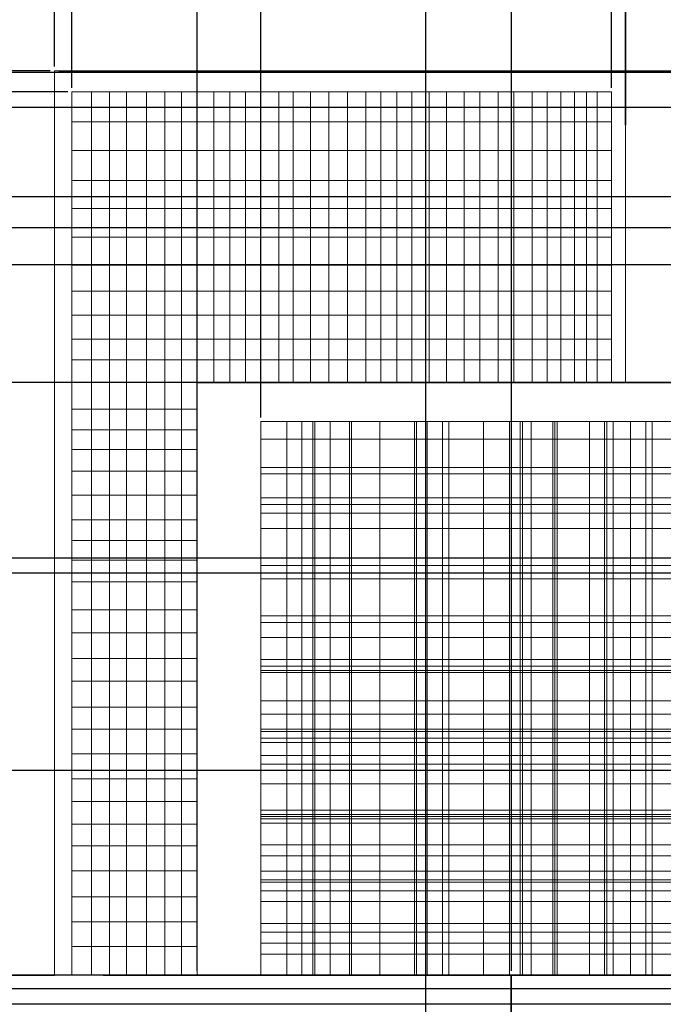
# Model space of a CAD drawing. Units: inches. Extents: x -10 to 130, y -32 to 34.
# Tile 7 of 22: x 19.07 to 28.66, y 5.57 to 20.25. Entities that reach past the tile are written whole.
import ezdxf

# ---------------------------------------------------------------- set-up
doc = ezdxf.new("R2010")
doc.units = ezdxf.units.IN
doc.header["$MEASUREMENT"] = 0
for name, color, linetype, lineweight in [('A-ANNO-DIMS', 2, 'Continuous', 18), ('A-ELEV', 7, 'Continuous', 35), ('A-GLAZ', 4, 'Continuous', 18)]:
    doc.layers.add(name, color=color, linetype=linetype, lineweight=lineweight)
doc.styles.get("Standard").update_dxf_attribs({"font": 'arial.ttf'})
doc.dimstyles.get("Standard").update_dxf_attribs({"dimtxt": 0.18, "dimasz": 0.18, "dimexe": 0.18, "dimexo": 0.0625, "dimgap": 0.09, "dimtad": 0, "dimtih": 1, "dimtoh": 1, "dimdec": 4, "dimzin": 0, "dimdsep": 46, "dimtxsty": 'Standard', "dimcen": 0.09, "dimadec": 0, "dimazin": 0, "dimtfac": 1, "dimtdec": 4, "dimtofl": 0, "dimtmove": 0, "dimatfit": 3, "dimfxl": 1, "dimtolj": 1, "dimtzin": 0, "dimarcsym": 0})

# ---------------------------------------------------------------- blocks, each defined once
blk = doc.blocks.new('*D3')
at = {"layer": 'A-ANNO-DIMS', "color": 0, "lineweight": -2, "transparency": 16777216}
for p, q in [((13.402, 6.07), (13.402, 33.879)), ((21.715, 6.07), (21.715, 33.879)), ((13.582, 33.699), (17.165, 33.699)), ((21.535, 33.699), (17.953, 33.699))]:
    blk.add_line(p, q, dxfattribs=at)
at = {"layer": 'A-ANNO-DIMS', "color": 0, "transparency": 16777216}
for points in [[(13.582, 33.729), (13.582, 33.669), (13.402, 33.699)], [(21.535, 33.729), (21.535, 33.669), (21.715, 33.699)]]:
    blk.add_solid(points, dxfattribs=at)
at = {"layer": 'Defpoints', "color": 0, "transparency": 16777216}
for p in [(21.715, 33.699), (13.402, 6.007), (21.715, 6.007)]:
    blk.add_point(p, dxfattribs=at)
at = {"layer": 'A-ANNO-DIMS', "color": 0, "transparency": 16777216, "insert": (17.559, 33.699), "char_height": 0.18, "attachment_point": 5}
blk.add_mtext('\\A1;8.313', dxfattribs=at)
blk = doc.blocks.new('*D4')
at = {"layer": 'A-ANNO-DIMS', "color": 0, "lineweight": -2, "transparency": 16777216}
for p, q in [((21.715, 6.07), (21.715, 33.879)), ((26.399, 6.07), (26.399, 33.879)), ((21.895, 33.699), (23.66, 33.699)), ((26.219, 33.699), (24.454, 33.699))]:
    blk.add_line(p, q, dxfattribs=at)
at = {"layer": 'A-ANNO-DIMS', "color": 0, "transparency": 16777216}
for points in [[(21.895, 33.729), (21.895, 33.669), (21.715, 33.699)], [(26.219, 33.729), (26.219, 33.669), (26.399, 33.699)]]:
    blk.add_solid(points, dxfattribs=at)
at = {"layer": 'Defpoints', "color": 0, "transparency": 16777216}
for p in [(26.399, 33.699), (21.715, 6.007), (26.399, 6.007)]:
    blk.add_point(p, dxfattribs=at)
at = {"layer": 'A-ANNO-DIMS', "color": 0, "transparency": 16777216, "insert": (24.057, 33.699), "char_height": 0.18, "attachment_point": 5}
blk.add_mtext('\\A1;4.683', dxfattribs=at)
blk = doc.blocks.new('*D5')
at = {"layer": 'A-ANNO-DIMS', "color": 0, "lineweight": -2, "transparency": 16777216}
for p, q in [((26.399, 6.07), (26.399, 33.879)), ((31.971, 6.07), (31.971, 33.879)), ((26.579, 33.699), (28.792, 33.699)), ((31.791, 33.699), (29.578, 33.699))]:
    blk.add_line(p, q, dxfattribs=at)
at = {"layer": 'A-ANNO-DIMS', "color": 0, "transparency": 16777216}
for points in [[(26.579, 33.729), (26.579, 33.669), (26.399, 33.699)], [(31.791, 33.729), (31.791, 33.669), (31.971, 33.699)]]:
    blk.add_solid(points, dxfattribs=at)
at = {"layer": 'Defpoints', "color": 0, "transparency": 16777216}
for p in [(31.971, 33.699), (26.399, 6.007), (31.971, 6.007)]:
    blk.add_point(p, dxfattribs=at)
at = {"layer": 'A-ANNO-DIMS', "color": 0, "transparency": 16777216, "insert": (29.185, 33.699), "char_height": 0.18, "attachment_point": 5}
blk.add_mtext('\\A1;5.572', dxfattribs=at)
blk = doc.blocks.new('*D11')
at = {"layer": 'A-ANNO-DIMS', "color": 0, "lineweight": -2, "transparency": 16777216}
for p, q in [((5.634, -12.739), (5.634, 33.879)), ((19.588, 19.547), (19.588, 33.879)), ((5.814, 33.699), (12.156, 33.699)), ((19.408, 33.699), (13.066, 33.699))]:
    blk.add_line(p, q, dxfattribs=at)
at = {"layer": 'A-ANNO-DIMS', "color": 0, "transparency": 16777216}
for points in [[(5.814, 33.729), (5.814, 33.669), (5.634, 33.699)], [(19.408, 33.729), (19.408, 33.669), (19.588, 33.699)]]:
    blk.add_solid(points, dxfattribs=at)
at = {"layer": 'Defpoints', "color": 0, "transparency": 16777216}
for p in [(19.588, 33.699), (19.588, 19.485), (5.634, -12.801)]:
    blk.add_point(p, dxfattribs=at)
at = {"layer": 'A-ANNO-DIMS', "color": 0, "transparency": 16777216, "insert": (12.611, 33.699), "char_height": 0.18, "attachment_point": 5}
blk.add_mtext('\\A1;13.954', dxfattribs=at)
blk = doc.blocks.new('*D12')
at = {"layer": 'A-ANNO-DIMS', "color": 0, "lineweight": -2, "transparency": 16777216}
for p, q in [((19.588, 19.547), (19.588, 33.879)), ((21.715, 14.903), (21.715, 33.879)), ((19.768, 33.699), (20.326, 33.699)), ((21.535, 33.699), (20.977, 33.699))]:
    blk.add_line(p, q, dxfattribs=at)
at = {"layer": 'A-ANNO-DIMS', "color": 0, "transparency": 16777216}
for points in [[(19.768, 33.729), (19.768, 33.669), (19.588, 33.699)], [(21.535, 33.729), (21.535, 33.669), (21.715, 33.699)]]:
    blk.add_solid(points, dxfattribs=at)
at = {"layer": 'Defpoints', "color": 0, "transparency": 16777216}
for p in [(21.715, 33.699), (19.588, 19.485), (21.715, 14.841)]:
    blk.add_point(p, dxfattribs=at)
at = {"layer": 'A-ANNO-DIMS', "color": 0, "transparency": 16777216, "insert": (20.652, 33.699), "char_height": 0.18, "attachment_point": 5}
blk.add_mtext('\\A1;2.13', dxfattribs=at)
blk = doc.blocks.new('*D13')
at = {"layer": 'A-ANNO-DIMS', "color": 0, "lineweight": -2, "transparency": 16777216}
for p, q in [((21.715, 14.903), (21.715, 33.879)), ((28.1, 24.464), (28.1, 33.879)), ((21.895, 33.699), (24.514, 33.699)), ((27.92, 33.699), (25.301, 33.699))]:
    blk.add_line(p, q, dxfattribs=at)
at = {"layer": 'A-ANNO-DIMS', "color": 0, "transparency": 16777216}
for points in [[(21.895, 33.729), (21.895, 33.669), (21.715, 33.699)], [(27.92, 33.729), (27.92, 33.669), (28.1, 33.699)]]:
    blk.add_solid(points, dxfattribs=at)
at = {"layer": 'Defpoints', "color": 0, "transparency": 16777216}
for p in [(28.1, 33.699), (28.1, 24.402), (21.715, 14.841)]:
    blk.add_point(p, dxfattribs=at)
at = {"layer": 'A-ANNO-DIMS', "color": 0, "transparency": 16777216, "insert": (24.908, 33.699), "char_height": 0.18, "attachment_point": 5}
blk.add_mtext('\\A1;6.384', dxfattribs=at)
blk = doc.blocks.new('*D14')
at = {"layer": 'A-ANNO-DIMS', "color": 0, "lineweight": -2, "transparency": 16777216}
for p, q in [((28.1, 24.464), (28.1, 33.879)), ((33.608, 19.52), (33.608, 33.879)), ((28.28, 33.699), (30.46, 33.699)), ((33.428, 33.699), (31.248, 33.699))]:
    blk.add_line(p, q, dxfattribs=at)
at = {"layer": 'A-ANNO-DIMS', "color": 0, "transparency": 16777216}
for points in [[(28.28, 33.729), (28.28, 33.669), (28.1, 33.699)], [(33.428, 33.729), (33.428, 33.669), (33.608, 33.699)]]:
    blk.add_solid(points, dxfattribs=at)
at = {"layer": 'Defpoints', "color": 0, "transparency": 16777216}
for p in [(33.608, 33.699), (28.1, 24.402), (33.608, 19.458)]:
    blk.add_point(p, dxfattribs=at)
at = {"layer": 'A-ANNO-DIMS', "color": 0, "transparency": 16777216, "insert": (30.854, 33.699), "char_height": 0.18, "attachment_point": 5}
blk.add_mtext('\\A1;5.508', dxfattribs=at)
blk = doc.blocks.new('*D28')
at = {"layer": 'A-ANNO-DIMS', "color": 0, "lineweight": -2, "transparency": 16777216}
for p, q in [((21.715, 14.903), (21.715, 33.879)), ((49.946, 14.903), (49.946, 33.879)), ((21.895, 33.699), (35.436, 33.699)), ((49.766, 33.699), (36.226, 33.699))]:
    blk.add_line(p, q, dxfattribs=at)
at = {"layer": 'A-ANNO-DIMS', "color": 0, "transparency": 16777216}
for points in [[(21.895, 33.729), (21.895, 33.669), (21.715, 33.699)], [(49.766, 33.729), (49.766, 33.669), (49.946, 33.699)]]:
    blk.add_solid(points, dxfattribs=at)
at = {"layer": 'Defpoints', "color": 0, "transparency": 16777216}
for p in [(49.946, 33.699), (21.715, 14.841), (49.946, 14.841)]:
    blk.add_point(p, dxfattribs=at)
at = {"layer": 'A-ANNO-DIMS', "color": 0, "transparency": 16777216, "insert": (35.831, 33.699), "char_height": 0.18, "attachment_point": 5}
blk.add_mtext('\\A1;28.23', dxfattribs=at)
blk = doc.blocks.new('*D34')
at = {"layer": 'A-ANNO-DIMS', "color": 0, "lineweight": -2, "transparency": 16777216}
for p, q in [((13.34, 6.007), (-9.564, 6.007)), ((-9.384, 5.827), (-9.384, 3.941)), ((-9.384, 1.691), (-9.384, 3.577)), ((70.835, 1.511), (-9.564, 1.511))]:
    blk.add_line(p, q, dxfattribs=at)
at = {"layer": 'A-ANNO-DIMS', "color": 0, "transparency": 16777216}
for points in [[(-9.414, 5.827), (-9.354, 5.827), (-9.384, 6.007)], [(-9.414, 1.691), (-9.354, 1.691), (-9.384, 1.511)]]:
    blk.add_solid(points, dxfattribs=at)
at = {"layer": 'Defpoints', "color": 0, "transparency": 16777216}
for p in [(-9.384, 6.007), (13.402, 6.007), (70.898, 1.511)]:
    blk.add_point(p, dxfattribs=at)
at = {"layer": 'A-ANNO-DIMS', "color": 0, "transparency": 16777216, "insert": (-9.384, 3.759), "char_height": 0.18, "attachment_point": 5}
blk.add_mtext('\\A1;4.497', dxfattribs=at)
blk = doc.blocks.new('*D35')
at = {"layer": 'A-ANNO-DIMS', "color": 0, "lineweight": -2, "transparency": 16777216}
for p, q in [((21.653, 14.841), (-9.564, 14.841)), ((-9.384, 14.661), (-9.384, 10.606)), ((-9.384, 6.187), (-9.384, 10.242)), ((13.34, 6.007), (-9.564, 6.007))]:
    blk.add_line(p, q, dxfattribs=at)
at = {"layer": 'A-ANNO-DIMS', "color": 0, "transparency": 16777216}
for points in [[(-9.414, 14.661), (-9.354, 14.661), (-9.384, 14.841)], [(-9.414, 6.187), (-9.354, 6.187), (-9.384, 6.007)]]:
    blk.add_solid(points, dxfattribs=at)
at = {"layer": 'Defpoints', "color": 0, "transparency": 16777216}
for p in [(-9.384, 14.841), (21.715, 14.841), (13.402, 6.007)]:
    blk.add_point(p, dxfattribs=at)
at = {"layer": 'A-ANNO-DIMS', "color": 0, "transparency": 16777216, "insert": (-9.384, 10.424), "char_height": 0.18, "attachment_point": 5}
blk.add_mtext('\\A1;8.833', dxfattribs=at)
blk = doc.blocks.new('*D36')
at = {"layer": 'A-ANNO-DIMS', "color": 0, "lineweight": -2, "transparency": 16777216}
for p, q in [((44.559, 17.607), (-9.564, 17.607)), ((-9.384, 17.427), (-9.384, 16.405)), ((-9.384, 15.021), (-9.384, 16.044)), ((21.653, 14.841), (-9.564, 14.841))]:
    blk.add_line(p, q, dxfattribs=at)
at = {"layer": 'A-ANNO-DIMS', "color": 0, "transparency": 16777216}
for points in [[(-9.414, 17.427), (-9.354, 17.427), (-9.384, 17.607)], [(-9.414, 15.021), (-9.354, 15.021), (-9.384, 14.841)]]:
    blk.add_solid(points, dxfattribs=at)
at = {"layer": 'Defpoints', "color": 0, "transparency": 16777216}
for p in [(-9.384, 17.607), (44.622, 17.607), (21.715, 14.841)]:
    blk.add_point(p, dxfattribs=at)
at = {"layer": 'A-ANNO-DIMS', "color": 0, "transparency": 16777216, "insert": (-9.384, 16.224), "char_height": 0.18, "attachment_point": 5}
blk.add_mtext('\\A1;2.77', dxfattribs=at)
blk = doc.blocks.new('*D37')
at = {"layer": 'A-ANNO-DIMS', "color": 0, "lineweight": -2, "transparency": 16777216}
for p, q in [((19.526, 19.485), (-9.564, 19.485)), ((-9.384, 19.305), (-9.384, 18.728)), ((-9.384, 17.787), (-9.384, 18.364)), ((44.559, 17.607), (-9.564, 17.607))]:
    blk.add_line(p, q, dxfattribs=at)
at = {"layer": 'A-ANNO-DIMS', "color": 0, "transparency": 16777216}
for points in [[(-9.414, 19.305), (-9.354, 19.305), (-9.384, 19.485)], [(-9.414, 17.787), (-9.354, 17.787), (-9.384, 17.607)]]:
    blk.add_solid(points, dxfattribs=at)
at = {"layer": 'Defpoints', "color": 0, "transparency": 16777216}
for p in [(-9.384, 19.485), (19.588, 19.485), (44.622, 17.607)]:
    blk.add_point(p, dxfattribs=at)
at = {"layer": 'A-ANNO-DIMS', "color": 0, "transparency": 16777216, "insert": (-9.384, 18.546), "char_height": 0.18, "attachment_point": 5}
blk.add_mtext('\\A1;1.877', dxfattribs=at)
blk = doc.blocks.new('*D38')
at = {"layer": 'A-ANNO-DIMS', "color": 0, "lineweight": -2, "transparency": 16777216}
for p, q in [((28.037, 24.402), (-9.564, 24.402)), ((-9.384, 24.222), (-9.384, 22.125)), ((-9.384, 19.665), (-9.384, 21.761)), ((19.526, 19.485), (-9.564, 19.485))]:
    blk.add_line(p, q, dxfattribs=at)
at = {"layer": 'A-ANNO-DIMS', "color": 0, "transparency": 16777216}
for points in [[(-9.414, 24.222), (-9.354, 24.222), (-9.384, 24.402)], [(-9.414, 19.665), (-9.354, 19.665), (-9.384, 19.485)]]:
    blk.add_solid(points, dxfattribs=at)
at = {"layer": 'Defpoints', "color": 0, "transparency": 16777216}
for p in [(-9.384, 24.402), (28.1, 24.402), (19.588, 19.485)]:
    blk.add_point(p, dxfattribs=at)
at = {"layer": 'A-ANNO-DIMS', "color": 0, "transparency": 16777216, "insert": (-9.384, 21.943), "char_height": 0.18, "attachment_point": 5}
blk.add_mtext('\\A1;4.917', dxfattribs=at)
blk = doc.blocks.new('*D74')
at = {"layer": 'A-ANNO-DIMS', "color": 0, "lineweight": -2, "transparency": 16777216}
for p, q in [((54.085, 17.607), (-9.564, 17.607)), ((-9.384, 17.427), (-9.384, 17.281)), ((-9.384, 16.771), (-9.384, 16.917)), ((55.856, 16.591), (-9.564, 16.591))]:
    blk.add_line(p, q, dxfattribs=at)
at = {"layer": 'A-ANNO-DIMS', "color": 0, "transparency": 16777216}
for points in [[(-9.414, 17.427), (-9.354, 17.427), (-9.384, 17.607)], [(-9.414, 16.771), (-9.354, 16.771), (-9.384, 16.591)]]:
    blk.add_solid(points, dxfattribs=at)
at = {"layer": 'Defpoints', "color": 0, "transparency": 16777216}
for p in [(54.147, 17.607), (-9.384, 16.591), (55.918, 16.591)]:
    blk.add_point(p, dxfattribs=at)
at = {"layer": 'A-ANNO-DIMS', "color": 0, "transparency": 16777216, "insert": (-9.384, 17.099), "char_height": 0.18, "attachment_point": 5}
blk.add_mtext('\\A1;1.02', dxfattribs=at)
blk = doc.blocks.new('*D82')
at = {"layer": 'A-ANNO-DIMS', "color": 0, "lineweight": -2, "transparency": 16777216}
for p, q in [((19.651, 19.485), (129.508, 19.485)), ((129.328, 19.305), (129.328, 18.728)), ((129.328, 17.787), (129.328, 18.364)), ((68.738, 17.607), (129.508, 17.607))]:
    blk.add_line(p, q, dxfattribs=at)
at = {"layer": 'A-ANNO-DIMS', "color": 0, "transparency": 16777216}
for points in [[(129.298, 19.305), (129.358, 19.305), (129.328, 19.485)], [(129.298, 17.787), (129.358, 17.787), (129.328, 17.607)]]:
    blk.add_solid(points, dxfattribs=at)
at = {"layer": 'Defpoints', "color": 0, "transparency": 16777216}
for p in [(19.588, 19.485), (68.676, 17.607), (129.328, 17.607)]:
    blk.add_point(p, dxfattribs=at)
at = {"layer": 'A-ANNO-DIMS', "color": 0, "transparency": 16777216, "insert": (129.328, 18.546), "char_height": 0.18, "attachment_point": 5}
blk.add_mtext('\\A1;1.877', dxfattribs=at)
blk = doc.blocks.new('*D87')
at = {"layer": 'A-ANNO-DIMS', "color": 0, "lineweight": -2, "transparency": 16777216}
for p, q in [((49.884, 14.841), (-9.564, 14.841)), ((-9.384, 14.661), (-9.384, 13.713)), ((-9.384, 12.402), (-9.384, 13.35)), ((49.884, 12.222), (-9.564, 12.222))]:
    blk.add_line(p, q, dxfattribs=at)
at = {"layer": 'A-ANNO-DIMS', "color": 0, "transparency": 16777216}
for points in [[(-9.414, 14.661), (-9.354, 14.661), (-9.384, 14.841)], [(-9.414, 12.402), (-9.354, 12.402), (-9.384, 12.222)]]:
    blk.add_solid(points, dxfattribs=at)
at = {"layer": 'Defpoints', "color": 0, "transparency": 16777216}
for p in [(49.946, 14.841), (-9.384, 12.222), (49.946, 12.222)]:
    blk.add_point(p, dxfattribs=at)
at = {"layer": 'A-ANNO-DIMS', "color": 0, "transparency": 16777216, "insert": (-9.384, 13.532), "char_height": 0.18, "attachment_point": 5}
blk.add_mtext('\\A1;2.619', dxfattribs=at)
blk = doc.blocks.new('*D88')
at = {"layer": 'A-ANNO-DIMS', "color": 0, "lineweight": -2, "transparency": 16777216}
for p, q in [((49.884, 12.222), (-9.564, 12.222)), ((-9.384, 12.042), (-9.384, 10.822)), ((-9.384, 9.238), (-9.384, 10.458)), ((49.884, 9.058), (-9.564, 9.058))]:
    blk.add_line(p, q, dxfattribs=at)
at = {"layer": 'A-ANNO-DIMS', "color": 0, "transparency": 16777216}
for points in [[(-9.414, 12.042), (-9.354, 12.042), (-9.384, 12.222)], [(-9.414, 9.238), (-9.354, 9.238), (-9.384, 9.058)]]:
    blk.add_solid(points, dxfattribs=at)
at = {"layer": 'Defpoints', "color": 0, "transparency": 16777216}
for p in [(49.946, 12.222), (-9.384, 9.058), (49.946, 9.058)]:
    blk.add_point(p, dxfattribs=at)
at = {"layer": 'A-ANNO-DIMS', "color": 0, "transparency": 16777216, "insert": (-9.384, 10.64), "char_height": 0.18, "attachment_point": 5}
blk.add_mtext('\\A1;3.164', dxfattribs=at)
blk = doc.blocks.new('*D89')
at = {"layer": 'A-ANNO-DIMS', "color": 0, "lineweight": -2, "transparency": 16777216}
for p, q in [((49.884, 9.058), (-9.564, 9.058)), ((-9.384, 8.878), (-9.384, 7.612)), ((-9.384, 5.982), (-9.384, 7.248)), ((49.884, 5.802), (-9.564, 5.802))]:
    blk.add_line(p, q, dxfattribs=at)
at = {"layer": 'A-ANNO-DIMS', "color": 0, "transparency": 16777216}
for points in [[(-9.414, 8.878), (-9.354, 8.878), (-9.384, 9.058)], [(-9.414, 5.982), (-9.354, 5.982), (-9.384, 5.802)]]:
    blk.add_solid(points, dxfattribs=at)
at = {"layer": 'Defpoints', "color": 0, "transparency": 16777216}
for p in [(49.946, 9.058), (-9.384, 5.802), (49.946, 5.802)]:
    blk.add_point(p, dxfattribs=at)
at = {"layer": 'A-ANNO-DIMS', "color": 0, "transparency": 16777216, "insert": (-9.384, 7.43), "char_height": 0.18, "attachment_point": 5}
blk.add_mtext('\\A1;3.256', dxfattribs=at)
blk = doc.blocks.new('*D90')
at = {"layer": 'A-ANNO-DIMS', "color": 0, "lineweight": -2, "transparency": 16777216}
for p, q in [((49.884, 5.802), (-9.564, 5.802)), ((-9.384, 5.622), (-9.384, 4.421)), ((-9.384, 2.855), (-9.384, 4.057)), ((49.884, 2.675), (-9.564, 2.675))]:
    blk.add_line(p, q, dxfattribs=at)
at = {"layer": 'A-ANNO-DIMS', "color": 0, "transparency": 16777216}
for points in [[(-9.414, 5.622), (-9.354, 5.622), (-9.384, 5.802)], [(-9.414, 2.855), (-9.354, 2.855), (-9.384, 2.675)]]:
    blk.add_solid(points, dxfattribs=at)
at = {"layer": 'Defpoints', "color": 0, "transparency": 16777216}
for p in [(49.946, 5.802), (-9.384, 2.675), (49.946, 2.675)]:
    blk.add_point(p, dxfattribs=at)
at = {"layer": 'A-ANNO-DIMS', "color": 0, "transparency": 16777216, "insert": (-9.384, 4.239), "char_height": 0.18, "attachment_point": 5}
blk.add_mtext('\\A1;3.127', dxfattribs=at)
blk = doc.blocks.new('*D95')
at = {"layer": 'A-ANNO-DIMS', "color": 0, "lineweight": -2, "transparency": 16777216}
for p, q in [((-9.384, 12.402), (-9.384, 12.582)), ((49.884, 12.222), (-9.564, 12.222)), ((49.884, 11.995), (-9.564, 11.995)), ((-9.384, 11.815), (-9.384, 11.635)), ((-9.384, 11.635), (-9.564, 11.635))]:
    blk.add_line(p, q, dxfattribs=at)
at = {"layer": 'A-ANNO-DIMS', "color": 0, "transparency": 16777216}
for points in [[(-9.414, 12.402), (-9.354, 12.402), (-9.384, 12.222)], [(-9.414, 11.815), (-9.354, 11.815), (-9.384, 11.995)]]:
    blk.add_solid(points, dxfattribs=at)
at = {"layer": 'Defpoints', "color": 0, "transparency": 16777216}
for p in [(49.946, 12.222), (-9.384, 11.995), (49.946, 11.995)]:
    blk.add_point(p, dxfattribs=at)
at = {"layer": 'A-ANNO-DIMS', "color": 0, "transparency": 16777216, "insert": (-9.957, 11.635), "char_height": 0.18, "attachment_point": 5}
blk.add_mtext('\\A1;0.227', dxfattribs=at)
blk = doc.blocks.new('*D96')
at = {"layer": 'A-ANNO-DIMS', "color": 0, "lineweight": -2, "transparency": 16777216}
for p, q in [((19.588, 19.547), (19.588, 33.879)), ((19.848, 19.232), (19.848, 33.879)), ((19.408, 33.699), (19.228, 33.699)), ((20.028, 33.699), (20.208, 33.699))]:
    blk.add_line(p, q, dxfattribs=at)
at = {"layer": 'A-ANNO-DIMS', "color": 0, "transparency": 16777216}
for points in [[(19.408, 33.729), (19.408, 33.669), (19.588, 33.699)], [(20.028, 33.729), (20.028, 33.669), (19.848, 33.699)]]:
    blk.add_solid(points, dxfattribs=at)
at = {"layer": 'Defpoints', "color": 0, "transparency": 16777216}
for p in [(19.848, 33.699), (19.588, 19.485), (19.848, 19.17)]:
    blk.add_point(p, dxfattribs=at)
at = {"layer": 'A-ANNO-DIMS', "color": 0, "transparency": 16777216, "insert": (20.601, 33.699), "char_height": 0.18, "attachment_point": 5}
blk.add_mtext('\\A1;0.260', dxfattribs=at)
blk = doc.blocks.new('*D97')
at = {"layer": 'A-ANNO-DIMS', "color": 0, "lineweight": -2, "transparency": 16777216}
for p, q in [((19.848, 19.232), (19.848, 33.879)), ((27.892, 19.232), (27.892, 33.879)), ((20.028, 33.699), (23.476, 33.699)), ((27.712, 33.699), (24.263, 33.699))]:
    blk.add_line(p, q, dxfattribs=at)
at = {"layer": 'A-ANNO-DIMS', "color": 0, "transparency": 16777216}
for points in [[(20.028, 33.729), (20.028, 33.669), (19.848, 33.699)], [(27.712, 33.729), (27.712, 33.669), (27.892, 33.699)]]:
    blk.add_solid(points, dxfattribs=at)
at = {"layer": 'Defpoints', "color": 0, "transparency": 16777216}
for p in [(27.892, 33.699), (19.848, 19.17), (27.892, 19.17)]:
    blk.add_point(p, dxfattribs=at)
at = {"layer": 'A-ANNO-DIMS', "color": 0, "transparency": 16777216, "insert": (23.87, 33.699), "char_height": 0.18, "attachment_point": 5}
blk.add_mtext('\\A1;8.044', dxfattribs=at)
blk = doc.blocks.new('*D98')
at = {"layer": 'A-ANNO-DIMS', "color": 0, "lineweight": -2, "transparency": 16777216}
for p, q in [((-9.384, 19.665), (-9.384, 19.845)), ((-9.384, 19.845), (-9.204, 19.845)), ((19.526, 19.485), (-9.564, 19.485)), ((19.785, 19.17), (-9.564, 19.17)), ((-9.384, 18.99), (-9.384, 18.81))]:
    blk.add_line(p, q, dxfattribs=at)
at = {"layer": 'A-ANNO-DIMS', "color": 0, "transparency": 16777216}
for points in [[(-9.414, 19.665), (-9.354, 19.665), (-9.384, 19.485)], [(-9.414, 18.99), (-9.354, 18.99), (-9.384, 19.17)]]:
    blk.add_solid(points, dxfattribs=at)
at = {"layer": 'Defpoints', "color": 0, "transparency": 16777216}
for p in [(-9.384, 19.485), (19.588, 19.485), (19.848, 19.17)]:
    blk.add_point(p, dxfattribs=at)
at = {"layer": 'A-ANNO-DIMS', "color": 0, "transparency": 16777216, "insert": (-8.809, 19.845), "char_height": 0.18, "attachment_point": 5}
blk.add_mtext('\\A1;0.315', dxfattribs=at)
blk = doc.blocks.new('*D104')
at = {"layer": 'A-ANNO-DIMS', "color": 0, "lineweight": -2, "transparency": 16777216}
for p, q in [((-9.383551, 19.637521), (-9.383551, 19.817521)), ((33.54566, 19.457521), (-9.563551, 19.457521)), ((33.931459, 18.935883), (-9.563551, 18.935883)), ((-9.383551, 18.755883), (-9.383551, 18.575883))]:
    blk.add_line(p, q, dxfattribs=at)
at = {"layer": 'A-ANNO-DIMS', "color": 0, "transparency": 16777216}
for points in [[(-9.413551, 19.637521), (-9.353551, 19.637521), (-9.383551, 19.457521)], [(-9.413551, 18.755883), (-9.353551, 18.755883), (-9.383551, 18.935883)]]:
    blk.add_solid(points, dxfattribs=at)
at = {"layer": 'Defpoints', "color": 0, "transparency": 16777216}
for p in [(-9.383551, 19.457521), (33.60816, 19.457521), (33.993959, 18.935883)]:
    blk.add_point(p, dxfattribs=at)
at = {"layer": 'A-ANNO-DIMS', "color": 0, "transparency": 16777216, "insert": (-9.383551, 19.196702), "char_height": 0.18, "attachment_point": 5}
blk.add_mtext('\\A1;0.522', dxfattribs=at)
blk = doc.blocks.new('*D105')
at = {"layer": 'A-ANNO-DIMS', "color": 0, "lineweight": -2, "transparency": 16777216}
for p, q in [((21.715452, 14.90344), (21.715452, 33.878656)), ((22.664856, 14.318095), (22.664856, 33.878656)), ((21.535452, 33.698656), (21.355452, 33.698656)), ((22.844856, 33.698656), (23.024856, 33.698656))]:
    blk.add_line(p, q, dxfattribs=at)
at = {"layer": 'A-ANNO-DIMS', "color": 0, "transparency": 16777216}
for points in [[(21.535452, 33.728656), (21.535452, 33.668656), (21.715452, 33.698656)], [(22.844856, 33.728656), (22.844856, 33.668656), (22.664856, 33.698656)]]:
    blk.add_solid(points, dxfattribs=at)
at = {"layer": 'Defpoints', "color": 0, "transparency": 16777216}
for p in [(22.664856, 33.698656), (21.715452, 14.84094), (22.664856, 14.255595)]:
    blk.add_point(p, dxfattribs=at)
at = {"layer": 'A-ANNO-DIMS', "color": 0, "transparency": 16777216, "insert": (22.190154, 33.698656), "char_height": 0.18, "attachment_point": 5}
blk.add_mtext('\\A1;0.949', dxfattribs=at)
blk = doc.blocks.new('*D106')
at = {"layer": 'A-ANNO-DIMS', "color": 0, "lineweight": -2, "transparency": 16777216}
for p, q in [((22.665, 14.318), (22.665, 33.879)), ((48.963, 14.318), (48.963, 33.879)), ((22.845, 33.699), (35.349, 33.699)), ((48.783, 33.699), (36.279, 33.699))]:
    blk.add_line(p, q, dxfattribs=at)
at = {"layer": 'A-ANNO-DIMS', "color": 0, "transparency": 16777216}
for points in [[(22.845, 33.729), (22.845, 33.669), (22.665, 33.699)], [(48.783, 33.729), (48.783, 33.669), (48.963, 33.699)]]:
    blk.add_solid(points, dxfattribs=at)
at = {"layer": 'Defpoints', "color": 0, "transparency": 16777216}
for p in [(48.963, 33.699), (22.665, 14.256), (48.963, 14.256)]:
    blk.add_point(p, dxfattribs=at)
at = {"layer": 'A-ANNO-DIMS', "color": 0, "transparency": 16777216, "insert": (35.814, 33.699), "char_height": 0.18, "attachment_point": 5}
blk.add_mtext('\\A1;26.298', dxfattribs=at)
blk = doc.blocks.new('*D110')
at = {"layer": 'A-ANNO-DIMS', "color": 0, "lineweight": -2, "transparency": 16777216}
for p, q in [((-9.383551, 17.787359), (-9.383551, 17.967359)), ((44.559228, 17.607359), (-9.563551, 17.607359)), ((45.040057, 17.142679), (-9.563551, 17.142679)), ((-9.383551, 16.962679), (-9.383551, 16.782679))]:
    blk.add_line(p, q, dxfattribs=at)
at = {"layer": 'A-ANNO-DIMS', "color": 0, "transparency": 16777216}
for points in [[(-9.413551, 17.787359), (-9.353551, 17.787359), (-9.383551, 17.607359)], [(-9.413551, 16.962679), (-9.353551, 16.962679), (-9.383551, 17.142679)]]:
    blk.add_solid(points, dxfattribs=at)
at = {"layer": 'Defpoints', "color": 0, "transparency": 16777216}
for p in [(-9.383551, 17.607359), (44.621728, 17.607359), (45.102557, 17.142679)]:
    blk.add_point(p, dxfattribs=at)
at = {"layer": 'A-ANNO-DIMS', "color": 0, "transparency": 16777216, "insert": (-9.383551, 17.375019), "char_height": 0.18, "attachment_point": 5}
blk.add_mtext('\\A1;0.465', dxfattribs=at)
blk = doc.blocks.new('*D112')
at = {"layer": 'A-ANNO-DIMS', "color": 0, "lineweight": -2, "transparency": 16777216}
for p, q in [((14.732, 5.012), (14.732, 33.879)), ((25.126, 5.012), (25.126, 33.879)), ((14.912, 33.699), (19.474, 33.699)), ((24.946, 33.699), (20.384, 33.699))]:
    blk.add_line(p, q, dxfattribs=at)
at = {"layer": 'A-ANNO-DIMS', "color": 0, "transparency": 16777216}
for points in [[(14.912, 33.729), (14.912, 33.669), (14.732, 33.699)], [(24.946, 33.729), (24.946, 33.669), (25.126, 33.699)]]:
    blk.add_solid(points, dxfattribs=at)
at = {"layer": 'Defpoints', "color": 0, "transparency": 16777216}
for p in [(25.126, 33.699), (14.732, 4.95), (25.126, 4.95)]:
    blk.add_point(p, dxfattribs=at)
at = {"layer": 'A-ANNO-DIMS', "color": 0, "transparency": 16777216, "insert": (19.929, 33.699), "char_height": 0.18, "attachment_point": 5}
blk.add_mtext('\\A1;10.394', dxfattribs=at)
blk = doc.blocks.new('*D115')
at = {"layer": 'A-ANNO-DIMS', "color": 0, "lineweight": -2, "transparency": 16777216}
for p, q in [((26.336, 6.007), (-9.564, 6.007)), ((-9.384, 5.827), (-9.384, 4.151)), ((-9.384, 2.111), (-9.384, 3.787)), ((26.336, 1.931), (-9.564, 1.931))]:
    blk.add_line(p, q, dxfattribs=at)
at = {"layer": 'A-ANNO-DIMS', "color": 0, "transparency": 16777216}
for points in [[(-9.414, 5.827), (-9.354, 5.827), (-9.384, 6.007)], [(-9.414, 2.111), (-9.354, 2.111), (-9.384, 1.931)]]:
    blk.add_solid(points, dxfattribs=at)
at = {"layer": 'Defpoints', "color": 0, "transparency": 16777216}
for p in [(26.399, 6.007), (-9.384, 1.931), (26.399, 1.931)]:
    blk.add_point(p, dxfattribs=at)
at = {"layer": 'A-ANNO-DIMS', "color": 0, "transparency": 16777216, "insert": (-9.384, 3.969), "char_height": 0.18, "attachment_point": 5}
blk.add_mtext('\\A1;4.076', dxfattribs=at)
blk = doc.blocks.new('*D121')
at = {"layer": 'A-ANNO-DIMS', "color": 0, "lineweight": -2, "transparency": 16777216}
for p, q in [((-9.384, 6.187), (-9.384, 6.367)), ((31.909, 6.007), (-9.564, 6.007)), ((32.427, 5.572), (-9.564, 5.572)), ((-9.384, 5.392), (-9.384, 5.212))]:
    blk.add_line(p, q, dxfattribs=at)
at = {"layer": 'A-ANNO-DIMS', "color": 0, "transparency": 16777216}
for points in [[(-9.414, 6.187), (-9.354, 6.187), (-9.384, 6.007)], [(-9.414, 5.392), (-9.354, 5.392), (-9.384, 5.572)]]:
    blk.add_solid(points, dxfattribs=at)
at = {"layer": 'Defpoints', "color": 0, "transparency": 16777216}
for p in [(-9.384, 6.007), (31.971, 6.007), (32.49, 5.572)]:
    blk.add_point(p, dxfattribs=at)
at = {"layer": 'A-ANNO-DIMS', "color": 0, "transparency": 16777216, "insert": (-9.384, 5.789), "char_height": 0.18, "attachment_point": 5}
blk.add_mtext('\\A1;0.436', dxfattribs=at)

msp = doc.modelspace()

# ---------------------------------------------------------------- linework, layer by layer
at = {"layer": 'A-ELEV'}
for p, q in [((28.0997, 18.6807), (28.0997, 24.4019)), ((21.7155, 14.8409), (49.9462, 14.8409)), ((19.5881, 6.0074), (13.4021, 6.0074)), ((20.3124, 6.0074), (49.9462, 6.0074)), ((26.3988, -6.2218), (26.3988, 6.0074))]:
    msp.add_line(p, q, dxfattribs=at)
at = {"layer": 'A-GLAZ'}
for p, q in [((20.3124, 19.4845), (19.5881, 19.4845)), ((19.5881, 19.4845), (19.5881, 18.6807)), ((20.3124, 19.4845), (28.0997, 19.4845)), ((19.8477, 19.1697), (27.8916, 19.1697)), ((19.8477, 19.1697), (19.8477, 18.6807)), ((20.1415, 19.1697), (20.1415, 18.6807)), ((20.408, 19.1697), (20.408, 18.6807)), ((20.6608, 19.1697), (20.6608, 18.6807)), ((20.9614, 19.1697), (20.9614, 18.6807)), ((21.2347, 19.1697), (21.2347, 18.6807)), ((21.4807, 19.1697), (21.4807, 18.6807)), ((21.7155, 14.8409), (21.7155, 19.1697)), ((21.9634, 14.8409), (21.9634, 19.1697)), ((22.2001, 14.8409), (22.2001, 19.1697)), ((22.4368, 14.8409), (22.4368, 19.1697)), ((22.6622, 14.8409), (22.6622, 19.1697)), ((22.9326, 14.8409), (22.9326, 19.1697)), ((23.1468, 14.8409), (23.1468, 19.1697)), ((23.406, 14.8409), (23.406, 19.1697)), ((23.6765, 14.8409), (23.6765, 19.1697)), ((23.9582, 14.8409), (23.9582, 19.1697)), ((24.2287, 14.8409), (24.2287, 19.1697)), ((24.4541, 14.8409), (24.4541, 19.1697)), ((24.6908, 14.8409), (24.6908, 19.1697)), ((24.9162, 14.8409), (24.9162, 19.1697)), ((25.1754, 14.8409), (25.1754, 19.1697)), ((25.4346, 14.8409), (25.4346, 19.1697)), ((25.6939, 14.8409), (25.6939, 19.1697)), ((25.9305, 14.8409), (25.9305, 19.1697)), ((26.201, 14.8409), (26.201, 19.1697)), ((26.4377, 14.8409), (26.4377, 19.1697)), ((26.7082, 14.8409), (26.7082, 19.1697)), ((26.9336, 14.8409), (26.9336, 19.1697)), ((27.1365, 14.8409), (27.1365, 19.1697)), ((27.3393, 14.8409), (27.3393, 19.1697)), ((27.5197, 14.8409), (27.5197, 19.1697)), ((27.6774, 14.8409), (27.6774, 19.1697)), ((27.8916, 14.8409), (27.8916, 19.1697)), ((19.5881, 18.6807), (19.5881, 6.7976)), ((19.8477, 18.7245), (27.8916, 18.7245)), ((19.8477, 18.6807), (19.8477, 6.7976)), ((20.1415, 18.6807), (20.1415, 6.7976)), ((20.408, 18.6807), (20.408, 6.7976)), ((20.6608, 18.6807), (20.6608, 6.7976)), ((20.9614, 18.6807), (20.9614, 6.7976)), ((21.2347, 18.6807), (21.2347, 6.7976)), ((21.4807, 18.6807), (21.4807, 6.7976)), ((28.0997, 18.6807), (28.0997, 14.8409)), ((20.3124, 18.2941), (19.8477, 18.2941)), ((20.3124, 18.2941), (27.8916, 18.2941)), ((20.3124, 17.8489), (19.8477, 17.8489)), ((20.3124, 17.8489), (27.8916, 17.8489)), ((20.3124, 17.4334), (19.8477, 17.4334)), ((20.3124, 17.4334), (27.8916, 17.4334)), ((20.3124, 17.0031), (19.8477, 17.0031)), ((20.3124, 17.0031), (27.8916, 17.0031)), ((20.3124, 16.5876), (19.8477, 16.5876)), ((20.3124, 16.5876), (27.8916, 16.5876)), ((20.3124, 16.1986), (19.8477, 16.1986)), ((20.3124, 16.1986), (27.8916, 16.1986)), ((20.3124, 15.8424), (19.8477, 15.8424)), ((20.3124, 15.8424), (27.8916, 15.8424)), ((20.3124, 15.4863), (19.8477, 15.4863)), ((20.3124, 15.4863), (27.8916, 15.4863)), ((20.3124, 15.1746), (19.8477, 15.1746)), ((20.3124, 15.1746), (27.8916, 15.1746)), ((21.7155, 14.8409), (19.8477, 14.8409)), ((21.7155, 6.0074), (21.7155, 14.8409)), ((20.3124, 14.4405), (19.8477, 14.4405)), ((20.3124, 14.4405), (21.7155, 14.4405)), ((22.6649, 6.0074), (22.6649, 14.2556)), ((22.6649, 14.2556), (48.963, 14.2556)), ((23.0516, 6.0074), (23.0516, 14.2556)), ((23.2772, 6.0074), (23.2772, 14.2556)), ((23.4383, 6.0074), (23.4383, 14.2556)), ((23.4706, 6.0074), (23.4706, 14.2556)), ((23.6962, 6.0074), (23.6962, 14.2556)), ((23.9862, 6.0074), (23.9862, 14.2556)), ((24.0184, 6.0074), (24.0184, 14.2556)), ((24.4374, 6.0074), (24.4374, 14.2556)), ((24.9531, 6.0074), (24.9531, 14.2556)), ((24.9853, 6.0074), (24.9853, 14.2556)), ((25.1464, 6.0074), (25.1464, 14.2556)), ((25.372, 6.0074), (25.372, 14.2556)), ((25.4687, 6.0074), (25.4687, 14.2556)), ((25.4687, 6.0074), (25.4687, 14.2556)), ((25.9844, 6.0074), (25.9844, 14.2556)), ((25.9844, 6.0074), (25.9844, 14.2556)), ((26.3711, 6.0074), (26.3711, 14.2556)), ((26.5322, 6.0074), (26.5322, 14.2556)), ((26.5645, 6.0074), (26.5645, 14.2556)), ((26.6934, 6.0074), (26.6934, 14.2556)), ((27.0156, 6.0074), (27.0156, 14.2556)), ((27.0479, 6.0074), (27.0479, 14.2556)), ((27.0801, 6.0074), (27.0801, 14.2556)), ((27.5635, 6.0074), (27.5635, 14.2556)), ((27.7891, 6.0074), (27.7891, 14.2556)), ((27.8214, 6.0074), (27.8214, 14.2556)), ((27.918, 6.0074), (27.918, 14.2556)), ((28.1759, 6.0074), (28.1759, 14.2556)), ((28.4015, 6.0074), (28.4015, 14.2556)), ((28.4981, 6.0074), (28.4981, 14.2556)), ((20.3124, 14.1324), (19.8477, 14.1324)), ((20.3124, 14.1324), (21.7155, 14.1324)), ((22.6649, 13.9954), (48.963, 13.9954)), ((20.3124, 13.8397), (19.8477, 13.8397)), ((20.3124, 13.8397), (21.7155, 13.8397)), ((20.3124, 13.5162), (19.8477, 13.5162)), ((20.3124, 13.5162), (21.7155, 13.5162)), ((22.6649, 13.5727), (48.963, 13.5727)), ((22.6649, 13.4751), (48.963, 13.4751)), ((20.3124, 13.1619), (19.8477, 13.1619)), ((20.3124, 13.1619), (21.7155, 13.1619)), ((22.6649, 13.1174), (48.963, 13.1174)), ((22.6649, 13.0199), (48.963, 13.0199)), ((20.3124, 12.7922), (19.8477, 12.7922)), ((20.3124, 12.7922), (21.7155, 12.7922)), ((22.6649, 12.8898), (48.963, 12.8898)), ((22.6649, 12.8898), (48.963, 12.8898)), ((22.6649, 12.6622), (48.963, 12.6622)), ((20.3124, 12.4841), (19.8477, 12.4841)), ((20.3124, 12.4841), (21.7155, 12.4841)), ((20.3124, 12.1914), (19.8477, 12.1914)), ((20.3124, 12.1914), (21.7155, 12.1914)), ((22.6649, 12.1093), (48.963, 12.1093)), ((22.6649, 11.9142), (48.963, 11.9142)), ((20.3124, 11.8679), (19.8477, 11.8679)), ((20.3124, 11.8679), (21.7155, 11.8679)), ((20.3124, 11.4484), (19.8477, 11.4484)), ((20.3124, 11.4484), (21.7155, 11.4484)), ((22.6649, 11.3614), (48.963, 11.3614)), ((22.6649, 11.3614), (48.963, 11.3614)), ((22.6649, 11.2638), (48.963, 11.2638)), ((20.3124, 11.1095), (19.8477, 11.1095)), ((20.3124, 11.1095), (21.7155, 11.1095)), ((22.6649, 11.0362), (48.963, 11.0362)), ((20.3124, 10.7244), (19.8477, 10.7244)), ((20.3124, 10.7244), (21.7155, 10.7244)), ((22.6649, 10.711), (48.963, 10.711)), ((22.6649, 10.711), (48.963, 10.711)), ((22.6649, 10.711), (48.963, 10.711)), ((22.6649, 10.6134), (48.963, 10.6134)), ((22.6649, 10.5484), (48.963, 10.5484)), ((22.6649, 10.5159), (48.963, 10.5159)), ((20.3124, 10.3855), (19.8477, 10.3855)), ((20.3124, 10.3855), (21.7155, 10.3855)), ((20.3124, 10.0004), (19.8477, 10.0004)), ((20.3124, 10.0004), (21.7155, 10.0004)), ((22.6649, 10.0931), (48.963, 10.0931)), ((22.6649, 9.898), (48.963, 9.898)), ((20.3124, 9.6726), (19.8477, 9.6726)), ((20.3124, 9.6726), (21.7155, 9.6726)), ((22.6649, 9.6704), (48.963, 9.6704)), ((22.6649, 9.6379), (48.963, 9.6379)), ((22.6649, 9.5403), (48.963, 9.5403)), ((22.6649, 9.4753), (48.963, 9.4753)), ((20.3124, 9.3028), (19.8477, 9.3028)), ((20.3124, 9.3028), (21.7155, 9.3028)), ((22.6649, 9.2802), (48.963, 9.2802)), ((22.6649, 9.1501), (48.963, 9.1501)), ((20.3124, 8.9331), (19.8477, 8.9331)), ((20.3124, 8.9331), (21.7155, 8.9331)), ((22.6649, 8.8574), (48.963, 8.8574)), ((20.3124, 8.5942), (19.8477, 8.5942)), ((20.3124, 8.5942), (21.7155, 8.5942)), ((22.6649, 8.4672), (48.963, 8.4672)), ((22.6649, 8.4021), (48.963, 8.4021)), ((22.6649, 8.3696), (48.963, 8.3696)), ((20.3124, 8.2553), (19.8477, 8.2553)), ((20.3124, 8.2553), (21.7155, 8.2553)), ((22.6649, 8.3371), (48.963, 8.3371)), ((22.6649, 8.2721), (48.963, 8.2721)), ((20.3124, 7.9319), (19.8477, 7.9319)), ((20.3124, 7.9319), (21.7155, 7.9319)), ((22.6649, 7.9469), (48.963, 7.9469)), ((22.6649, 7.7843), (48.963, 7.7843)), ((20.3124, 7.5621), (19.8477, 7.5621)), ((20.3124, 7.5621), (21.7155, 7.5621)), ((22.6649, 7.5566), (48.963, 7.5566)), ((22.6649, 7.4266), (48.963, 7.4266)), ((22.6649, 7.3941), (48.963, 7.3941)), ((22.6649, 7.264), (48.963, 7.264)), ((20.3124, 7.1718), (19.8477, 7.1718)), ((20.3124, 7.1718), (21.7155, 7.1718)), ((22.6649, 7.1014), (48.963, 7.1014)), ((19.5881, 6.0074), (19.5881, 6.7976)), ((20.3124, 6.8021), (19.8477, 6.8021)), ((19.8477, 6.0074), (19.8477, 6.7976)), ((20.1415, 6.0074), (20.1415, 6.7976)), ((20.3124, 6.8021), (21.7155, 6.8021)), ((20.408, 6.0074), (20.408, 6.7976)), ((20.6608, 6.0074), (20.6608, 6.7976)), ((20.9614, 6.0074), (20.9614, 6.7976)), ((21.2347, 6.0074), (21.2347, 6.7976)), ((21.4807, 6.0074), (21.4807, 6.7976)), ((22.6649, 6.7762), (48.963, 6.7762)), ((22.6649, 6.6461), (48.963, 6.6461)), ((22.6649, 6.4835), (48.963, 6.4835)), ((20.3124, 6.4324), (19.8477, 6.4324)), ((20.3124, 6.4324), (21.7155, 6.4324)), ((22.6649, 6.3209), (48.963, 6.3209)), ((20.3124, 6.0074), (19.5881, 6.0074))]:
    msp.add_line(p, q, dxfattribs=at)

# ---------------------------------------------------------------- dimensions: what is measured, and where the dimension line sits
at = {"layer": 'A-ANNO-DIMS'}
for base, p1, p2, override, picture, middle in [((19.5881, 33.6987), (5.634, -12.8012), (19.5881, 19.4845), {"dimdec": 3, "dimlfac": 1, "dimrnd": 0, "dimzin": 0, "dimdsep": 46, "dimlunit": 2}, '*D11', (12.611, 33.6987)), ((21.7155, 33.6987), (13.4021, 6.0074), (21.7155, 6.0074), {"dimdec": 3, "dimlfac": 1, "dimrnd": 0, "dimzin": 0, "dimdsep": 46, "dimlunit": 2}, '*D3', (17.5588, 33.6987)), ((25.1261, 33.6987), (14.7324, 4.9495), (25.1261, 4.9495), {"dimdec": 3, "dimlfac": 1, "dimrnd": 0, "dimzin": 0, "dimdsep": 46, "dimlunit": 2}, '*D112', (19.9293, 33.6987)), ((19.8477, 33.6987), (19.5881, 19.4845), (19.8477, 19.1697), {"dimdec": 3, "dimlfac": 1, "dimrnd": 0, "dimzin": 0, "dimdsep": 46, "dimlunit": 2}, '*D96', (20.6011, 33.6987)), ((21.7155, 33.6987), (19.5881, 19.4845), (21.7155, 14.8409), {"dimdec": 2, "dimlfac": 1, "dimrnd": 0, "dimzin": 0, "dimdsep": 46, "dimlunit": 2}, '*D12', (20.6518, 33.6987)), ((27.8916, 33.6987), (19.8477, 19.1697), (27.8916, 19.1697), {"dimdec": 3, "dimlfac": 1, "dimrnd": 0, "dimzin": 0, "dimdsep": 46, "dimlunit": 2}, '*D97', (23.8696, 33.6987)), ((22.6649, 33.6987), (21.7155, 14.8409), (22.6649, 14.2556), {"dimdec": 3, "dimlfac": 1, "dimrnd": 0, "dimzin": 0, "dimdsep": 46, "dimlunit": 2}, '*D105', (22.1902, 33.6987)), ((26.3988, 33.6987), (21.7155, 6.0074), (26.3988, 6.0074), {"dimdec": 3, "dimlfac": 1, "dimrnd": 0, "dimzin": 0, "dimdsep": 46, "dimlunit": 2}, '*D4', (24.0571, 33.6987)), ((28.0997, 33.6987), (21.7155, 14.8409), (28.0997, 24.4019), {"dimdec": 3, "dimlfac": 1, "dimrnd": 0, "dimzin": 0, "dimdsep": 46, "dimlunit": 2}, '*D13', (24.9076, 33.6987)), ((49.9462, 33.6987), (21.7155, 14.8409), (49.9462, 14.8409), {"dimdec": 2, "dimlfac": 1, "dimrnd": 0, "dimzin": 0, "dimdsep": 46, "dimlunit": 2}, '*D28', (35.8308, 33.6987)), ((48.963, 33.6987), (22.6649, 14.2556), (48.963, 14.2556), {"dimdec": 3, "dimlfac": 1, "dimrnd": 0, "dimzin": 0, "dimdsep": 46, "dimlunit": 2}, '*D106', (35.8139, 33.6987)), ((31.9712, 33.6987), (26.3988, 6.0074), (31.9712, 6.0074), {"dimdec": 3, "dimlfac": 1, "dimrnd": 0, "dimzin": 0, "dimdsep": 46, "dimlunit": 2}, '*D5', (29.185, 33.6987)), ((33.60816, 33.69866), (28.0997, 24.40191), (33.60816, 19.45752), {"dimdec": 3, "dimlfac": 1, "dimrnd": 0, "dimzin": 0, "dimdsep": 46, "dimlunit": 2}, '*D14', (30.85393, 33.69866))]:
    dim = msp.add_linear_dim(base=base, p1=p1, p2=p2, dimstyle='Standard', override=override, dxfattribs=at)
    dim.commit()
    dim.dimension.update_dxf_attribs({"geometry": picture, "text_midpoint": middle})
for base, p1, p2, override, picture, middle in [((-9.3836, 24.4019), (19.5881, 19.4845), (28.0997, 24.4019), {"dimdec": 3, "dimlfac": 1, "dimrnd": 0, "dimzin": 0, "dimdsep": 46, "dimlunit": 2}, '*D38', (-9.3836, 21.9432)), ((-9.3836, 19.4845), (19.8477, 19.1697), (19.5881, 19.4845), {"dimdec": 3, "dimlfac": 1, "dimrnd": 0, "dimzin": 0, "dimdsep": 46, "dimlunit": 2}, '*D98', (-8.8092, 19.8445)), ((-9.3836, 19.4575), (33.994, 18.9359), (33.6082, 19.4575), {"dimdec": 3, "dimlfac": 1, "dimrnd": 0, "dimzin": 0, "dimdsep": 46, "dimlunit": 2}, '*D104', (-9.3836, 19.1967)), ((-9.3836, 19.4845), (44.6217, 17.6074), (19.5881, 19.4845), {"dimdec": 3, "dimlfac": 1, "dimrnd": 0, "dimzin": 0, "dimdsep": 46, "dimlunit": 2}, '*D37', (-9.3836, 18.5459)), ((129.3277, 17.6074), (19.5881, 19.4845), (68.6759, 17.6074), {"dimdec": 3, "dimlfac": 1, "dimrnd": 0, "dimzin": 0, "dimdsep": 46, "dimlunit": 2}, '*D82', (129.3277, 18.5459)), ((-9.3836, 17.6074), (45.1026, 17.1427), (44.6217, 17.6074), {"dimdec": 3, "dimlfac": 1, "dimrnd": 0, "dimzin": 0, "dimdsep": 46, "dimlunit": 2}, '*D110', (-9.3836, 17.375)), ((-9.3836, 17.6074), (21.7155, 14.8409), (44.6217, 17.6074), {"dimdec": 2, "dimlfac": 1, "dimrnd": 0, "dimzin": 0, "dimdsep": 46, "dimlunit": 2}, '*D36', (-9.3836, 16.2241)), ((-9.3836, 16.5911), (54.1471, 17.6074), (55.9182, 16.5911), {"dimdec": 2, "dimlfac": 1, "dimrnd": 0, "dimzin": 0, "dimdsep": 46, "dimlunit": 2}, '*D74', (-9.3836, 17.0992)), ((-9.383551, 14.84094), (13.402105, 6.007442), (21.715452, 14.84094), {"dimdec": 3, "dimlfac": 1, "dimrnd": 0, "dimzin": 0, "dimdsep": 46, "dimlunit": 2}, '*D35', (-9.383551, 10.424191)), ((-9.3836, 12.2222), (49.9462, 14.8409), (49.9462, 12.2222), {"dimdec": 3, "dimlfac": 1, "dimrnd": 0, "dimzin": 0, "dimdsep": 46, "dimlunit": 2}, '*D87', (-9.3836, 13.5316)), ((-9.3836, 11.9951), (49.9462, 12.2222), (49.9462, 11.9951), {"dimdec": 3, "dimlfac": 1, "dimrnd": 0, "dimzin": 0, "dimdsep": 46, "dimlunit": 2}, '*D95', (-9.9573, 11.6351)), ((-9.3836, 9.058), (49.9462, 12.2222), (49.9462, 9.058), {"dimdec": 3, "dimlfac": 1, "dimrnd": 0, "dimzin": 0, "dimdsep": 46, "dimlunit": 2}, '*D88', (-9.3836, 10.6401)), ((-9.3836, 5.8024), (49.9462, 9.058), (49.9462, 5.8024), {"dimdec": 3, "dimlfac": 1, "dimrnd": 0, "dimzin": 0, "dimdsep": 46, "dimlunit": 2}, '*D89', (-9.3836, 7.4302)), ((-9.3836, 6.0074), (32.4898, 5.5715), (31.9712, 6.0074), {"dimdec": 3, "dimlfac": 1, "dimrnd": 0, "dimzin": 0, "dimdsep": 46, "dimlunit": 2}, '*D121', (-9.3836, 5.7895)), ((-9.3836, 6.0074), (70.898, 1.5107), (13.4021, 6.0074), {"dimdec": 3, "dimlfac": 1, "dimrnd": 0, "dimzin": 0, "dimdsep": 46, "dimlunit": 2}, '*D34', (-9.3836, 3.7591)), ((-9.3836, 1.931), (26.3988, 6.0074), (26.3988, 1.931), {"dimdec": 3, "dimlfac": 1, "dimrnd": 0, "dimzin": 0, "dimdsep": 46, "dimlunit": 2}, '*D115', (-9.3836, 3.9692)), ((-9.3836, 2.6753), (49.9462, 5.8024), (49.9462, 2.6753), {"dimdec": 3, "dimlfac": 1, "dimrnd": 0, "dimzin": 0, "dimdsep": 46, "dimlunit": 2}, '*D90', (-9.3836, 4.2388))]:
    dim = msp.add_linear_dim(base=base, p1=p1, p2=p2, angle=90, dimstyle='Standard', override=override, dxfattribs=at)
    dim.commit()
    dim.dimension.update_dxf_attribs({"geometry": picture, "text_midpoint": middle})

doc.saveas('drawing.dxf')
